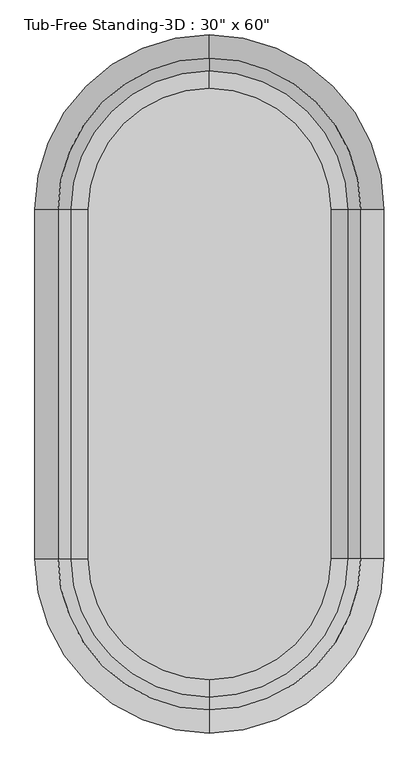
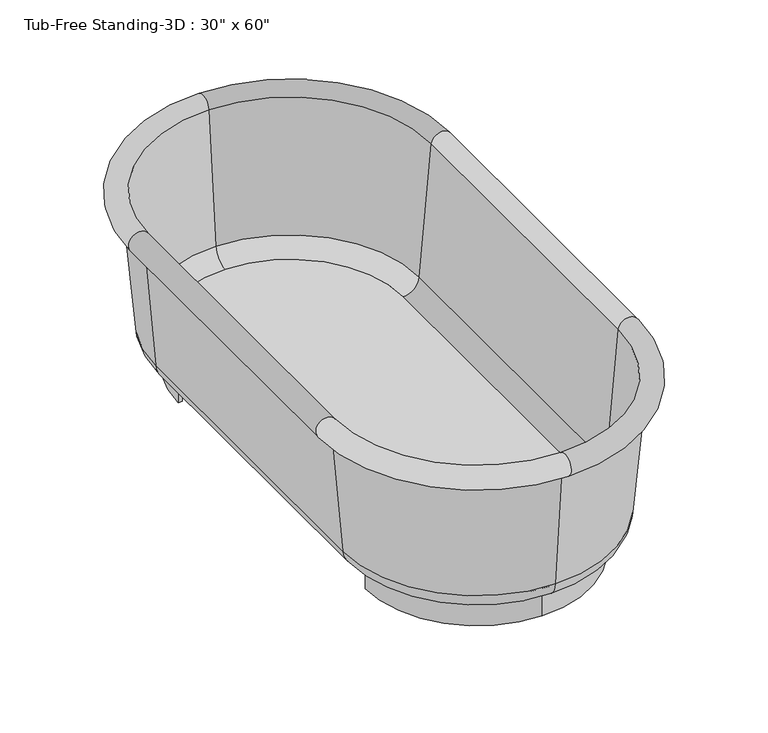
"""IFC4 building model written with IfcOpenShell, lengths in millimetres: flow terminal geometry."""

from ifc_helpers import new_model, si_unit, point, frame, frame_2d, origin, origin_with_axes, place, context, project, spatial, polyline, circle_curve, ellipse_curve, trimmed, segment, composite_curve, outline, extrude, source, transform, mapped, element, save
from ifc_brep_helpers import plane_surface, cylinder_surface, revolved_surface, advanced_brep


def flow_terminal_f2f0329d(model_context):
    return source(origin(), model_context, "Body", "SolidModel", [
        extrude(outline(composite_curve([segment(trimmed(circle_curve(frame_2d((0.0, -381.0)), 254.0), [point((0.0, -635.0))], [point((254.0, -381.0))], True, "CARTESIAN"), True, "CONTINUOUS"), segment(polyline([(254.0, -381.0), (264.2824236, -381.0)]), True, "CONTINUOUS"), segment(trimmed(circle_curve(frame_2d((0.0, -381.0)), 264.2824236), [point((264.2824236, -381.0))], [point((0.0, -645.2824236))], False, "CARTESIAN"), True, "CONTINUOUS"), segment(trimmed(circle_curve(frame_2d((0.0, -381.0)), 264.2824236), [point((0.0, -645.2824236))], [point((-264.2824236, -381.0))], False, "CARTESIAN"), True, "CONTINUOUS"), segment(polyline([(-264.2824236, -381.0), (-254.0, -381.0)]), True, "CONTINUOUS"), segment(trimmed(circle_curve(frame_2d((0.0, -381.0)), 254.0), [point((-254.0, -381.0))], [point((0.0, -635.0))], True, "CARTESIAN"), True, "CONTINUOUS")], self_intersect=False)), origin_with_axes(), (0.0, 0.0, 1.0), 63.5),
        extrude(outline(composite_curve([segment(trimmed(circle_curve(frame_2d((0.0, 381.0)), 264.2824236), [point((0.0, 645.2824236))], [point((264.2824236, 381.0))], False, "CARTESIAN"), True, "CONTINUOUS"), segment(polyline([(264.2824236, 381.0), (254.0, 381.0)]), True, "CONTINUOUS"), segment(trimmed(circle_curve(frame_2d((0.0, 381.0)), 254.0), [point((254.0, 381.0))], [point((0.0, 635.0))], True, "CARTESIAN"), True, "CONTINUOUS"), segment(trimmed(circle_curve(frame_2d((0.0, 381.0)), 254.0), [point((0.0, 635.0))], [point((-254.0, 381.0))], True, "CARTESIAN"), True, "CONTINUOUS"), segment(polyline([(-254.0, 381.0), (-264.2824236, 381.0)]), True, "CONTINUOUS"), segment(trimmed(circle_curve(frame_2d((0.0, 381.0)), 264.2824236), [point((-264.2824236, 381.0))], [point((0.0, 645.2824236))], False, "CARTESIAN"), True, "CONTINUOUS")], self_intersect=False)), origin_with_axes(), (0.0, 0.0, 1.0), 63.5),
        extrude(outline(composite_curve([segment(trimmed(circle_curve(frame_2d((0.0, 381.0)), 264.2824236), [point((-264.2824236, 381.0))], [point((0.0, 645.2824236))], False, "CARTESIAN"), True, "CONTINUOUS"), segment(trimmed(circle_curve(frame_2d((0.0, 381.0)), 264.2824236), [point((0.0, 645.2824236))], [point((264.2824236, 381.0))], False, "CARTESIAN"), True, "CONTINUOUS"), segment(polyline([(264.2824236, 381.0), (264.2824236, -381.0)]), True, "CONTINUOUS"), segment(trimmed(circle_curve(frame_2d((0.0, -381.0)), 264.2824236), [point((264.2824236, -381.0))], [point((0.0, -645.2824236))], False, "CARTESIAN"), True, "CONTINUOUS"), segment(trimmed(circle_curve(frame_2d((0.0, -381.0)), 264.2824236), [point((0.0, -645.2824236))], [point((-264.2824236, -381.0))], False, "CARTESIAN"), True, "CONTINUOUS"), segment(polyline([(-264.2824236, -381.0), (-264.2824236, 381.0)]), True, "CONTINUOUS")], self_intersect=False)), frame((0.0, 0.0, 63.5), z_axis=(0.0, 0.0, 1.0), x_axis=(1.0, 0.0, 0.0)), (0.0, 0.0, 1.0), 15.08125),
        advanced_brep(
        [(0.0, 723.9, 406.4), (0.0, 736.6, 406.4), (355.6, 381.0, 406.4), (342.9, 381.0, 406.4), (0.0, 698.1045038, 111.5561295), (317.1045038, 381.0, 111.5561295), (0.0, 645.2824236, 63.1536107), (264.2824236, 381.0, 63.1536107), (0.0, 645.2824236, 78.0774627), (264.2824236, 381.0, 78.0774627), (0.0, 683.2374416, 112.8568289), (302.2374416, 381.0, 112.8568289), (0.0, 711.4561556, 435.3982063), (330.4561556, 381.0, 435.3982063), (-342.9, 381.0, 406.4), (-355.6, 381.0, 406.4), (-317.1045038, 381.0, 111.5561295), (-264.2824236, 381.0, 63.1536107), (-264.2824236, 381.0, 78.0774627), (-302.2374416, 381.0, 112.8568289), (-330.4561556, 381.0, 435.3982063), (-342.9, -381.0, 406.4), (-355.6, -381.0, 406.4), (-317.1045038, -381.0, 111.5561295), (-264.2824236, -381.0, 63.1536107), (-264.2824236, -381.0, 78.0774627), (-302.2374416, -381.0, 112.8568289), (-330.4561556, -381.0, 435.3982063), (0.0, -723.9, 406.4), (0.0, -736.6, 406.4), (0.0, -698.1045038, 111.5561295), (0.0, -645.2824236, 63.1536107), (0.0, -645.2824236, 78.0774627), (0.0, -683.2374416, 112.8568289), (0.0, -711.4561556, 435.3982063), (342.9, -381.0, 406.4), (355.6, -381.0, 406.4), (317.1045038, -381.0, 111.5561295), (264.2824236, -381.0, 63.1536107), (264.2824236, -381.0, 78.0774627), (302.2374416, -381.0, 112.8568289), (330.4561556, -381.0, 435.3982063)],
        [
            (0, 1),
            (1, 2, circle_curve(frame((0.0, 381.0, 406.4), z_axis=(0.0, 0.0, -1.0), x_axis=(1.0, 0.0, 0.0)), 355.6)),
            (2, 3),
            (3, 0, circle_curve(frame((0.0, 381.0, 406.4), z_axis=(0.0, 0.0, 1.0), x_axis=(1.0, 0.0, 0.0)), 342.9)),
            (4, 0),
            (3, 5),
            (5, 4, circle_curve(frame((0.0, 381.0, 111.5561295), z_axis=(0.0, 0.0, 1.0), x_axis=(1.0, 0.0, 0.0)), 317.1045038)),
            (6, 4, circle_curve(frame((0.0, 645.2824236, 116.1774627), z_axis=(1.0, 0.0, 0.0), x_axis=(0.0, 1.0, 0.0)), 53.023852)),
            (5, 7, circle_curve(frame((264.2824236, 381.0, 116.1774627), z_axis=(0.0, 1.0, 0.0), x_axis=(1.0, 0.0, 0.0)), 53.023852)),
            (7, 6, circle_curve(frame((0.0, 381.0, 63.1536107), z_axis=(0.0, 0.0, 1.0), x_axis=(1.0, 0.0, 0.0)), 264.2824236)),
            (8, 6),
            (7, 9),
            (9, 8, circle_curve(frame((0.0, 381.0, 78.0774627), z_axis=(0.0, 0.0, 1.0), x_axis=(1.0, 0.0, 0.0)), 264.2824236)),
            (10, 8, circle_curve(frame((0.0, 645.2824236, 116.1774627), z_axis=(-1.0, 0.0, 0.0), x_axis=(0.0, 1.0, 0.0)), 38.1)),
            (9, 11, circle_curve(frame((264.2824236, 381.0, 116.1774627), z_axis=(0.0, -1.0, 0.0), x_axis=(1.0, 0.0, 0.0)), 38.1)),
            (11, 10, circle_curve(frame((0.0, 381.0, 112.8568289), z_axis=(0.0, 0.0, 1.0), x_axis=(1.0, 0.0, 0.0)), 302.2374416)),
            (12, 10),
            (11, 13),
            (13, 12, circle_curve(frame((0.0, 381.0, 435.3982063), z_axis=(0.0, 0.0, 1.0), x_axis=(1.0, 0.0, 0.0)), 330.4561556)),
            (1, 12, circle_curve(frame((0.0, 736.6, 431.8), z_axis=(1.0, 0.0, 0.0), x_axis=(0.0, 1.0, 0.0)), 25.4)),
            (13, 2, circle_curve(frame((355.6, 381.0, 431.8), z_axis=(0.0, 1.0, 0.0), x_axis=(1.0, 0.0, 0.0)), 25.4)),
            (14, 15),
            (15, 1, circle_curve(frame((0.0, 381.0, 406.4), z_axis=(0.0, 0.0, -1.0), x_axis=(0.0, 1.0, 0.0)), 355.6)),
            (0, 14, circle_curve(frame((0.0, 381.0, 406.4), z_axis=(0.0, 0.0, 1.0), x_axis=(0.0, 1.0, 0.0)), 342.9)),
            (16, 14),
            (4, 16, circle_curve(frame((0.0, 381.0, 111.5561295), z_axis=(0.0, 0.0, 1.0), x_axis=(0.0, 1.0, 0.0)), 317.1045038)),
            (17, 16, circle_curve(frame((-264.2824236, 381.0, 116.1774627), z_axis=(0.0, 1.0, 0.0), x_axis=(-1.0, 0.0, 0.0)), 53.023852)),
            (6, 17, circle_curve(frame((0.0, 381.0, 63.1536107), z_axis=(0.0, 0.0, 1.0), x_axis=(0.0, 1.0, 0.0)), 264.2824236)),
            (18, 17),
            (8, 18, circle_curve(frame((0.0, 381.0, 78.0774627), z_axis=(0.0, 0.0, 1.0), x_axis=(0.0, 1.0, 0.0)), 264.2824236)),
            (19, 18, circle_curve(frame((-264.2824236, 381.0, 116.1774627), z_axis=(0.0, -1.0, 0.0), x_axis=(-1.0, 0.0, 0.0)), 38.1)),
            (10, 19, circle_curve(frame((0.0, 381.0, 112.8568289), z_axis=(0.0, 0.0, 1.0), x_axis=(0.0, 1.0, 0.0)), 302.2374416)),
            (20, 19),
            (12, 20, circle_curve(frame((0.0, 381.0, 435.3982063), z_axis=(0.0, 0.0, 1.0), x_axis=(0.0, 1.0, 0.0)), 330.4561556)),
            (15, 20, circle_curve(frame((-355.6, 381.0, 431.8), z_axis=(0.0, 1.0, 0.0), x_axis=(-1.0, 0.0, 0.0)), 25.4)),
            (14, 21),
            (21, 22),
            (22, 15),
            (16, 23),
            (23, 21),
            (17, 24),
            (24, 23, circle_curve(frame((-264.2824236, -381.0, 116.1774627), z_axis=(0.0, 1.0, 0.0), x_axis=(-1.0, 0.0, 0.0)), 53.023852)),
            (18, 25),
            (25, 24),
            (19, 26),
            (26, 25, circle_curve(frame((-264.2824236, -381.0, 116.1774627), z_axis=(0.0, -1.0, 0.0), x_axis=(-1.0, 0.0, 0.0)), 38.1)),
            (20, 27),
            (27, 26),
            (22, 27, circle_curve(frame((-355.6, -381.0, 431.8), z_axis=(0.0, 1.0, 0.0), x_axis=(-1.0, 0.0, 0.0)), 25.4)),
            (28, 29),
            (29, 22, circle_curve(frame((0.0, -381.0, 406.4), z_axis=(0.0, 0.0, -1.0), x_axis=(-1.0, 0.0, 0.0)), 355.6)),
            (21, 28, circle_curve(frame((0.0, -381.0, 406.4), z_axis=(0.0, 0.0, 1.0), x_axis=(-1.0, 0.0, 0.0)), 342.9)),
            (30, 28),
            (23, 30, circle_curve(frame((0.0, -381.0, 111.5561295), z_axis=(0.0, 0.0, 1.0), x_axis=(-1.0, 0.0, 0.0)), 317.1045038)),
            (31, 30, circle_curve(frame((0.0, -645.2824236, 116.1774627), z_axis=(-1.0, 0.0, 0.0), x_axis=(0.0, -1.0, 0.0)), 53.023852)),
            (24, 31, circle_curve(frame((0.0, -381.0, 63.1536107), z_axis=(0.0, 0.0, 1.0), x_axis=(-1.0, 0.0, 0.0)), 264.2824236)),
            (32, 31),
            (25, 32, circle_curve(frame((0.0, -381.0, 78.0774627), z_axis=(0.0, 0.0, 1.0), x_axis=(-1.0, 0.0, 0.0)), 264.2824236)),
            (33, 32, circle_curve(frame((0.0, -645.2824236, 116.1774627), z_axis=(1.0, 0.0, 0.0), x_axis=(0.0, -1.0, 0.0)), 38.1)),
            (26, 33, circle_curve(frame((0.0, -381.0, 112.8568289), z_axis=(0.0, 0.0, 1.0), x_axis=(-1.0, 0.0, 0.0)), 302.2374416)),
            (34, 33),
            (27, 34, circle_curve(frame((0.0, -381.0, 435.3982063), z_axis=(0.0, 0.0, 1.0), x_axis=(-1.0, 0.0, 0.0)), 330.4561556)),
            (29, 34, circle_curve(frame((0.0, -736.6, 431.8), z_axis=(-1.0, 0.0, 0.0), x_axis=(0.0, -1.0, 0.0)), 25.4)),
            (35, 36),
            (36, 29, circle_curve(frame((0.0, -381.0, 406.4), z_axis=(0.0, 0.0, -1.0), x_axis=(0.0, -1.0, 0.0)), 355.6)),
            (28, 35, circle_curve(frame((0.0, -381.0, 406.4), z_axis=(0.0, 0.0, 1.0), x_axis=(0.0, -1.0, 0.0)), 342.9)),
            (37, 35),
            (30, 37, circle_curve(frame((0.0, -381.0, 111.5561295), z_axis=(0.0, 0.0, 1.0), x_axis=(0.0, -1.0, 0.0)), 317.1045038)),
            (38, 37, circle_curve(frame((264.2824236, -381.0, 116.1774627), z_axis=(0.0, -1.0, 0.0), x_axis=(1.0, 0.0, 0.0)), 53.023852)),
            (31, 38, circle_curve(frame((0.0, -381.0, 63.1536107), z_axis=(0.0, 0.0, 1.0), x_axis=(0.0, -1.0, 0.0)), 264.2824236)),
            (39, 38),
            (32, 39, circle_curve(frame((0.0, -381.0, 78.0774627), z_axis=(0.0, 0.0, 1.0), x_axis=(0.0, -1.0, 0.0)), 264.2824236)),
            (40, 39, circle_curve(frame((264.2824236, -381.0, 116.1774627), z_axis=(0.0, 1.0, 0.0), x_axis=(1.0, 0.0, 0.0)), 38.1)),
            (33, 40, circle_curve(frame((0.0, -381.0, 112.8568289), z_axis=(0.0, 0.0, 1.0), x_axis=(0.0, -1.0, 0.0)), 302.2374416)),
            (41, 40),
            (34, 41, circle_curve(frame((0.0, -381.0, 435.3982063), z_axis=(0.0, 0.0, 1.0), x_axis=(0.0, -1.0, 0.0)), 330.4561556)),
            (36, 41, circle_curve(frame((355.6, -381.0, 431.8), z_axis=(0.0, -1.0, 0.0), x_axis=(1.0, 0.0, 0.0)), 25.4)),
            (35, 3),
            (2, 36),
            (37, 5),
            (38, 7),
            (39, 9),
            (40, 11),
            (41, 13),
        ],
        [
            plane_surface(frame((0.0, 381.0, 406.4), z_axis=(0.0, 0.0, -1.0), x_axis=(1.0, 0.0, 0.0))),
            revolved_surface(polyline([(342.9, 381.0, 406.4), (317.1045038, 381.0, 111.5561295)]), (0.0, 381.0, 431.8), (0.0, 0.0, -1.0)),
            revolved_surface(trimmed(ellipse_curve(frame((264.2824236, 381.0, 116.1774627), z_axis=(0.0, 1.0, 0.0), x_axis=(1.0, 0.0, 0.0)), 53.023852, 53.023852), [point((317.1045038, 381.0, 111.5561295))], [point((264.2824236, 381.0, 63.1536107))], True, "CARTESIAN"), (0.0, 381.0, 431.8), (0.0, 0.0, -1.0)),
            revolved_surface(polyline([(264.2824236, 381.0, 63.1536107), (264.2824236, 381.0, 78.07746270000001)]), (0.0, 381.0, 431.8), (0.0, 0.0, -1.0)),
            revolved_surface(trimmed(ellipse_curve(frame((264.2824236, 381.0, 116.1774627), z_axis=(0.0, -1.0, 0.0), x_axis=(1.0, 0.0, 0.0)), 38.1, 38.1), [point((264.2824236, 381.0, 78.0774627))], [point((302.2374416, 381.0, 112.8568289))], True, "CARTESIAN"), (0.0, 381.0, 431.8), (0.0, 0.0, -1.0)),
            revolved_surface(polyline([(302.2374416, 381.0, 112.8568289), (330.4561556, 381.0, 435.3982063)]), (0.0, 381.0, 431.8), (0.0, 0.0, -1.0)),
            revolved_surface(trimmed(ellipse_curve(frame((355.6, 381.0, 431.8), z_axis=(0.0, 1.0, 0.0), x_axis=(1.0, 0.0, 0.0)), 25.4, 25.4), [point((330.4561556, 381.0, 435.3982063))], [point((355.6, 381.0, 406.4))], True, "CARTESIAN"), (0.0, 381.0, 431.8), (0.0, 0.0, -1.0)),
            plane_surface(frame((0.0, 381.0, 406.4), z_axis=(0.0, 0.0, -1.0), x_axis=(0.0, 1.0, 0.0))),
            revolved_surface(polyline([(0.0, 723.9, 406.4), (0.0, 698.1045038, 111.5561295)]), (0.0, 381.0, 431.8), (0.0, 0.0, -1.0)),
            revolved_surface(trimmed(ellipse_curve(frame((0.0, 645.2824236, 116.1774627), z_axis=(-1.0, 0.0, 0.0), x_axis=(0.0, 1.0, 0.0)), 53.023852, 53.023852), [point((0.0, 698.1045038, 111.5561295))], [point((0.0, 645.2824236, 63.1536107))], True, "CARTESIAN"), (0.0, 381.0, 431.8), (0.0, 0.0, -1.0)),
            revolved_surface(polyline([(0.0, 645.2824236, 63.1536107), (0.0, 645.2824236, 78.07746270000001)]), (0.0, 381.0, 431.8), (0.0, 0.0, -1.0)),
            revolved_surface(trimmed(ellipse_curve(frame((0.0, 645.2824236, 116.1774627), z_axis=(1.0, 0.0, 0.0), x_axis=(0.0, 1.0, 0.0)), 38.1, 38.1), [point((0.0, 645.2824236, 78.0774627))], [point((0.0, 683.2374416, 112.8568289))], True, "CARTESIAN"), (0.0, 381.0, 431.8), (0.0, 0.0, -1.0)),
            revolved_surface(polyline([(0.0, 683.2374416, 112.8568289), (0.0, 711.4561556, 435.3982063)]), (0.0, 381.0, 431.8), (0.0, 0.0, -1.0)),
            revolved_surface(trimmed(ellipse_curve(frame((0.0, 736.6, 431.8), z_axis=(-1.0, 0.0, 0.0), x_axis=(0.0, 1.0, 0.0)), 25.4, 25.4), [point((0.0, 711.4561556, 435.3982063))], [point((0.0, 736.6, 406.4))], True, "CARTESIAN"), (0.0, 381.0, 431.8), (0.0, 0.0, -1.0)),
            plane_surface(frame((-355.6, 381.0, 406.4), z_axis=(0.0, 0.0, -1.0), x_axis=(0.0, -1.0, 0.0))),
            plane_surface(frame((-342.9, 381.0, 406.4), z_axis=(-0.9961946980917455, 0.0, -0.08715574274765871), x_axis=(0.0, -1.0, 0.0))),
            cylinder_surface(frame((-264.2824236, 381.0, 116.1774627), z_axis=(0.0, 1.0, 0.0), x_axis=(-1.0, 0.0, 0.0)), 53.023852),
            plane_surface(frame((-264.2824236, 381.0, 63.1536107), z_axis=(1.0, 0.0, 0.0), x_axis=(0.0, -1.0, 0.0))),
            revolved_surface(polyline([(-302.38242360000004, -381.0, 116.1774627), (-302.38242360000004, 381.0, 116.1774627)]), (-264.2824236, 381.0, 116.1774627), (0.0, -1.0, 0.0)),
            plane_surface(frame((-302.2374416, 381.0, 112.8568289), z_axis=(0.9961946980917458, 0.0, 0.08715574274765651), x_axis=(0.0, -1.0, 0.0))),
            cylinder_surface(frame((-355.6, 381.0, 431.8), z_axis=(0.0, 1.0, 0.0), x_axis=(-1.0, 0.0, 0.0)), 25.4),
            plane_surface(frame((0.0, -381.0, 406.4), z_axis=(0.0, 0.0, -1.0), x_axis=(-1.0, 0.0, 0.0))),
            revolved_surface(polyline([(-342.9, -381.0, 406.4), (-317.1045038, -381.0, 111.5561295)]), (0.0, -381.0, 431.8), (0.0, 0.0, -1.0)),
            revolved_surface(trimmed(ellipse_curve(frame((-264.2824236, -381.0, 116.1774627), z_axis=(0.0, -1.0, 0.0), x_axis=(-1.0, 0.0, 0.0)), 53.023852, 53.023852), [point((-317.1045038, -381.0, 111.5561295))], [point((-264.2824236, -381.0, 63.1536107))], True, "CARTESIAN"), (0.0, -381.0, 431.8), (0.0, 0.0, -1.0)),
            revolved_surface(polyline([(-264.2824236, -381.0, 63.1536107), (-264.2824236, -381.0, 78.07746270000001)]), (0.0, -381.0, 431.8), (0.0, 0.0, -1.0)),
            revolved_surface(trimmed(ellipse_curve(frame((-264.2824236, -381.0, 116.1774627), z_axis=(0.0, 1.0, 0.0), x_axis=(-1.0, 0.0, 0.0)), 38.1, 38.1), [point((-264.2824236, -381.0, 78.0774627))], [point((-302.2374416, -381.0, 112.8568289))], True, "CARTESIAN"), (0.0, -381.0, 431.8), (0.0, 0.0, -1.0)),
            revolved_surface(polyline([(-302.2374416, -381.0, 112.8568289), (-330.4561556, -381.0, 435.3982063)]), (0.0, -381.0, 431.8), (0.0, 0.0, -1.0)),
            revolved_surface(trimmed(ellipse_curve(frame((-355.6, -381.0, 431.8), z_axis=(0.0, -1.0, 0.0), x_axis=(-1.0, 0.0, 0.0)), 25.4, 25.4), [point((-330.4561556, -381.0, 435.3982063))], [point((-355.6, -381.0, 406.4))], True, "CARTESIAN"), (0.0, -381.0, 431.8), (0.0, 0.0, -1.0)),
            plane_surface(frame((0.0, -381.0, 406.4), z_axis=(0.0, 0.0, -1.0), x_axis=(0.0, -1.0, 0.0))),
            revolved_surface(polyline([(0.0, -723.9, 406.4), (0.0, -698.1045038, 111.5561295)]), (0.0, -381.0, 431.8), (0.0, 0.0, -1.0)),
            revolved_surface(trimmed(ellipse_curve(frame((0.0, -645.2824236, 116.1774627), z_axis=(1.0, 0.0, 0.0), x_axis=(0.0, -1.0, 0.0)), 53.023852, 53.023852), [point((0.0, -698.1045038, 111.5561295))], [point((0.0, -645.2824236, 63.1536107))], True, "CARTESIAN"), (0.0, -381.0, 431.8), (0.0, 0.0, -1.0)),
            revolved_surface(polyline([(0.0, -645.2824236, 63.1536107), (0.0, -645.2824236, 78.07746270000001)]), (0.0, -381.0, 431.8), (0.0, 0.0, -1.0)),
            revolved_surface(trimmed(ellipse_curve(frame((0.0, -645.2824236, 116.1774627), z_axis=(-1.0, 0.0, 0.0), x_axis=(0.0, -1.0, 0.0)), 38.1, 38.1), [point((0.0, -645.2824236, 78.0774627))], [point((0.0, -683.2374416, 112.8568289))], True, "CARTESIAN"), (0.0, -381.0, 431.8), (0.0, 0.0, -1.0)),
            revolved_surface(polyline([(0.0, -683.2374416, 112.8568289), (0.0, -711.4561556, 435.3982063)]), (0.0, -381.0, 431.8), (0.0, 0.0, -1.0)),
            revolved_surface(trimmed(ellipse_curve(frame((0.0, -736.6, 431.8), z_axis=(1.0, 0.0, 0.0), x_axis=(0.0, -1.0, 0.0)), 25.4, 25.4), [point((0.0, -711.4561556, 435.3982063))], [point((0.0, -736.6, 406.4))], True, "CARTESIAN"), (0.0, -381.0, 431.8), (0.0, 0.0, -1.0)),
            plane_surface(frame((355.6, -381.0, 406.4), z_axis=(0.0, 0.0, -1.0), x_axis=(0.0, 1.0, 0.0))),
            plane_surface(frame((342.9, -381.0, 406.4), z_axis=(0.9961946980917455, 0.0, -0.08715574274765871), x_axis=(0.0, 1.0, 0.0))),
            cylinder_surface(frame((264.2824236, -381.0, 116.1774627), z_axis=(0.0, -1.0, 0.0), x_axis=(1.0, 0.0, 0.0)), 53.023852),
            plane_surface(frame((264.2824236, -381.0, 63.1536107), z_axis=(-1.0, 0.0, 0.0), x_axis=(0.0, 1.0, 0.0))),
            revolved_surface(polyline([(302.38242360000004, 381.0, 116.1774627), (302.38242360000004, -381.0, 116.1774627)]), (264.2824236, -381.0, 116.1774627), (0.0, 1.0, 0.0)),
            plane_surface(frame((302.2374416, -381.0, 112.8568289), z_axis=(-0.9961946980917458, 0.0, 0.08715574274765651), x_axis=(0.0, 1.0, 0.0))),
            cylinder_surface(frame((355.6, -381.0, 431.8), z_axis=(0.0, -1.0, 0.0), x_axis=(1.0, 0.0, 0.0)), 25.4),
        ],
        [
            (0, [[1, 2, 3, 4]]),
            (1, [[5, -4, 6, 7]]),
            (2, [[8, -7, 9, 10]]),
            (3, [[11, -10, 12, 13]]),
            (4, [[14, -13, 15, 16]]),
            (5, [[17, -16, 18, 19]]),
            (6, [[20, -19, 21, -2]]),
            (7, [[22, 23, -1, 24]]),
            (8, [[25, -24, -5, 26]]),
            (9, [[27, -26, -8, 28]]),
            (10, [[29, -28, -11, 30]]),
            (11, [[31, -30, -14, 32]]),
            (12, [[33, -32, -17, 34]]),
            (13, [[35, -34, -20, -23]]),
            (14, [[36, 37, 38, -22]]),
            (15, [[39, 40, -36, -25]]),
            (16, [[41, 42, -39, -27]]),
            (17, [[43, 44, -41, -29]]),
            (18, [[45, 46, -43, -31]]),
            (19, [[47, 48, -45, -33]]),
            (20, [[-38, 49, -47, -35]]),
            (21, [[50, 51, -37, 52]]),
            (22, [[53, -52, -40, 54]]),
            (23, [[55, -54, -42, 56]]),
            (24, [[57, -56, -44, 58]]),
            (25, [[59, -58, -46, 60]]),
            (26, [[61, -60, -48, 62]]),
            (27, [[63, -62, -49, -51]]),
            (28, [[64, 65, -50, 66]]),
            (29, [[67, -66, -53, 68]]),
            (30, [[69, -68, -55, 70]]),
            (31, [[71, -70, -57, 72]]),
            (32, [[73, -72, -59, 74]]),
            (33, [[75, -74, -61, 76]]),
            (34, [[77, -76, -63, -65]]),
            (35, [[78, -3, 79, -64]]),
            (36, [[80, -6, -78, -67]]),
            (37, [[81, -9, -80, -69]]),
            (38, [[82, -12, -81, -71]]),
            (39, [[83, -15, -82, -73]]),
            (40, [[84, -18, -83, -75]]),
            (41, [[-79, -21, -84, -77]]),
        ],
    ),
    ])


if __name__ == "__main__":
    model = new_model("IFC4")
    model_context = context("Model", 3, world=origin())
    ifc_project = project(units=[si_unit("LENGTHUNIT", "METRE", prefix="MILLI")], contexts=[model_context])
    site = spatial("IfcSite", under=ifc_project)
    building = spatial("IfcBuilding", under=site)
    placement = place(None, origin())
    flow_terminal_shape = flow_terminal_f2f0329d(model_context)
    element("IfcFlowTerminal", 1, ObjectType="Tub-Free Standing-3D : 30\" x 60\"", at=placement, inside=building, context=model_context, shape_type="MappedRepresentation", body=[
        mapped(flow_terminal_shape, transform((0.0, 0.0, 0.0), x_axis=(1.0, 0.0, 0.0), y_axis=(0.0, 1.0, 0.0), z_axis=(0.0, 0.0, 1.0))),
    ])
    save(model, "model.ifc")

# Revit data of these elements
# Type "Tub-Free Standing-3D : 30\" x 60\""
#   Assembly Code = "D2010110"
#   Height = 1' - 6"
#   Length = 5' - 0"
#   Width = 2' - 6"
#   Tub Material = Porcelain, Ivory
#   Default Elevation = 0
# Element 1 (IfcFlowTerminal, "Tub-Free Standing-3D : 30\" x 60\"")
#   Materials on its faces: "Porcelain, Ivory"
# Materials
#   "Porcelain, Ivory": class "Ceramic", colour RGB 247 247 239, transparency 0, Description = "Porcelain, ivory", Cost = 0
